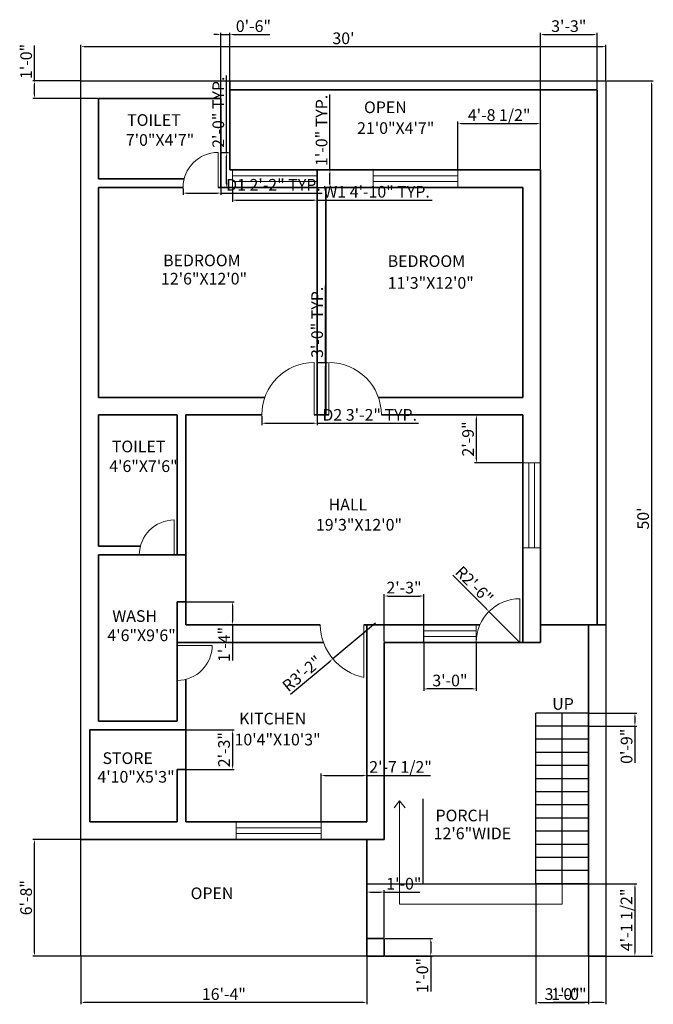
# Model space of a CAD drawing. Units: inches. Extents: x 2514 to 2949, y 1604 to 2279.
import ezdxf

# ---------------------------------------------------------------- set-up
doc = ezdxf.new("R2010")
doc.units = ezdxf.units.IN
for name, color, linetype, lineweight in [('A-ANNO-DIMS', 7, 'Continuous', 18), ('A-ANNO-SYMB', 121, 'Continuous', 18), ('A-ANNO-TEXT', 231, 'Continuous', 18), ('A-AREA-IDEN', 231, 'Continuous', 18), ('A-COLS', 121, 'Continuous', 35), ('A-DOOR', 2, 'Continuous', 18), ('A-FLOR-STRS', 121, 'Continuous', 25), ('A-GLAZ', 40, 'Continuous', 18), ('A-WALL', 121, 'Continuous', 35), ('C-PROP', 121, 'Continuous', 25)]:
    doc.layers.add(name, color=color, linetype=linetype, lineweight=lineweight)
doc.styles.get("Standard").update_dxf_attribs({"font": 'arial.ttf'})
doc.dimstyles.new('ISO-25', dxfattribs={"dimtxt": 8, "dimasz": 2.5, "dimexe": 1.25, "dimexo": 0.625, "dimtad": 1, "dimdec": 0, "dimlunit": 3, "dimtxsty": 'Standard', "dimcen": 2.5, "dimadec": 0, "dimazin": 0, "dimtfac": 1, "dimtdec": 0, "dimtmove": 0, "dimatfit": 3, "dimfxl": 1, "dimarcsym": 0})

# ---------------------------------------------------------------- blocks, each defined once
blk = doc.blocks.new('*D1')
at = {"layer": 'A-ANNO-DIMS', "color": 0, "lineweight": -2, "transparency": 16777216}
for p, q in [((2556.32, 2237.43), (2556.32, 2261.58)), ((2558.82, 2260.33), (2913.82, 2260.33)), ((2916.32, 2237.43), (2916.32, 2261.58))]:
    blk.add_line(p, q, dxfattribs=at)
at = {"layer": 'A-ANNO-DIMS', "color": 0, "transparency": 16777216}
for points in [[(2558.82, 2260.74), (2558.82, 2259.91), (2556.32, 2260.33)], [(2913.82, 2260.74), (2913.82, 2259.91), (2916.32, 2260.33)]]:
    blk.add_solid(points, dxfattribs=at)
at = {"layer": 'Defpoints', "color": 0, "transparency": 16777216}
for p in [(2916.32, 2260.33), (2556.32, 2236.8), (2916.32, 2236.8)]:
    blk.add_point(p, dxfattribs=at)
at = {"layer": 'A-ANNO-DIMS', "color": 0, "transparency": 16777216, "insert": (2736.32, 2265.04), "char_height": 8, "attachment_point": 5}
blk.add_mtext("30'", dxfattribs=at)
blk = doc.blocks.new('*D2')
at = {"layer": 'A-ANNO-DIMS', "color": 0, "lineweight": -2, "transparency": 16777216}
for p, q in [((2916.94, 2236.8), (2948.78, 2236.8)), ((2947.53, 2234.3), (2947.53, 1639.3)), ((2916.94, 1636.8), (2948.78, 1636.8))]:
    blk.add_line(p, q, dxfattribs=at)
at = {"layer": 'A-ANNO-DIMS', "color": 0, "transparency": 16777216}
for points in [[(2947.11, 2234.3), (2947.95, 2234.3), (2947.53, 2236.8)], [(2947.11, 1639.3), (2947.95, 1639.3), (2947.53, 1636.8)]]:
    blk.add_solid(points, dxfattribs=at)
at = {"layer": 'Defpoints', "color": 0, "transparency": 16777216}
for p in [(2916.32, 2236.8), (2916.32, 1636.8), (2947.53, 1636.8)]:
    blk.add_point(p, dxfattribs=at)
at = {"layer": 'A-ANNO-DIMS', "color": 0, "transparency": 16777216, "insert": (2942.82, 1936.8), "char_height": 8, "attachment_point": 5, "rotation": 90}
blk.add_mtext("50'", dxfattribs=at)
blk = doc.blocks.new('DOOR-SWING-24IN')
for p, q in [((0, 0), (0, 24)), ((2, 0), (0, 0))]:
    blk.add_line(p, q)
blk.add_arc((0, 0), 24, 90, 180)
blk = doc.blocks.new('DOOR-SWING-36IN')
for p, q in [((0, 0), (0, 36)), ((2, 0), (0, 0))]:
    blk.add_line(p, q)
blk.add_arc((0, 0), 36, 90, 180)
blk = doc.blocks.new('WIN-WIDE-12IN-WALL')
for p, q in [((0, 12), (0, 0)), ((0, 8), (58.18, 8)), ((58.18, 0), (58.18, 12)), ((0, 4), (58.18, 4))]:
    blk.add_line(p, q)
blk = doc.blocks.new('STAIR-TREAD-36IN')
for p, q in [((18, 0), (0, 0)), ((36, 0), (18, 0))]:
    blk.add_line(p, q)
blk = doc.blocks.new('*D7')
at = {"layer": 'A-ANNO-DIMS', "color": 0, "lineweight": -2, "transparency": 16777216}
for p, q in [((2660.14, 2163.18), (2660.14, 2153.83)), ((2718.32, 2163.18), (2718.32, 2153.83)), ((2662.64, 2155.08), (2715.82, 2155.08)), ((2718.32, 2155.08), (2797.24, 2155.08))]:
    blk.add_line(p, q, dxfattribs=at)
at = {"layer": 'A-ANNO-DIMS', "color": 0, "transparency": 16777216}
for points in [[(2662.64, 2155.49), (2662.64, 2154.66), (2660.14, 2155.08)], [(2715.82, 2155.49), (2715.82, 2154.66), (2718.32, 2155.08)]]:
    blk.add_solid(points, dxfattribs=at)
at = {"layer": 'Defpoints', "color": 0, "transparency": 16777216}
for p in [(2660.14, 2163.8), (2718.32, 2163.8), (2718.32, 2155.08)]:
    blk.add_point(p, dxfattribs=at)
at = {"layer": 'A-ANNO-DIMS', "color": 0, "transparency": 16777216, "insert": (2759.03, 2159.79), "char_height": 8, "attachment_point": 5}
blk.add_mtext('W1 4\'-10" TYP.', dxfattribs=at)
blk = doc.blocks.new('*D8')
at = {"layer": 'A-ANNO-DIMS', "color": 0, "lineweight": -2, "transparency": 16777216}
for p, q in [((2727.04, 2175.8), (2727.04, 2227.56)), ((2718.94, 2175.8), (2728.29, 2175.8)), ((2727.04, 2166.3), (2727.04, 2173.3)), ((2718.94, 2163.8), (2728.29, 2163.8))]:
    blk.add_line(p, q, dxfattribs=at)
at = {"layer": 'A-ANNO-DIMS', "color": 0, "transparency": 16777216}
for points in [[(2726.62, 2173.3), (2727.46, 2173.3), (2727.04, 2175.8)], [(2726.62, 2166.3), (2727.46, 2166.3), (2727.04, 2163.8)]]:
    blk.add_solid(points, dxfattribs=at)
at = {"layer": 'Defpoints', "color": 0, "transparency": 16777216}
for p in [(2718.32, 2175.8), (2727.04, 2175.8), (2718.32, 2163.8)]:
    blk.add_point(p, dxfattribs=at)
at = {"layer": 'A-ANNO-DIMS', "color": 0, "transparency": 16777216, "insert": (2722.33, 2202.93), "char_height": 8, "attachment_point": 5, "rotation": 90}
blk.add_mtext('1\'-0" TYP.', dxfattribs=at)
blk = doc.blocks.new('*D9')
at = {"layer": 'A-ANNO-DIMS', "color": 0, "lineweight": -2, "transparency": 16777216}
for p, q in [((2626.32, 2163.18), (2626.32, 2158.65)), ((2652.32, 2163.18), (2652.32, 2158.65)), ((2628.82, 2159.9), (2649.82, 2159.9)), ((2652.32, 2159.9), (2721.82, 2159.9))]:
    blk.add_line(p, q, dxfattribs=at)
at = {"layer": 'A-ANNO-DIMS', "color": 0, "transparency": 16777216}
for points in [[(2628.82, 2160.32), (2628.82, 2159.49), (2626.32, 2159.9)], [(2649.82, 2160.32), (2649.82, 2159.49), (2652.32, 2159.9)]]:
    blk.add_solid(points, dxfattribs=at)
at = {"layer": 'Defpoints', "color": 0, "transparency": 16777216}
for p in [(2626.32, 2163.8), (2652.32, 2163.8), (2652.32, 2159.9)]:
    blk.add_point(p, dxfattribs=at)
at = {"layer": 'A-ANNO-DIMS', "color": 0, "transparency": 16777216, "insert": (2688.32, 2164.55), "char_height": 8, "attachment_point": 5}
blk.add_mtext('D1 2\'-2" TYP.', dxfattribs=at)
blk = doc.blocks.new('*D10')
at = {"layer": 'A-ANNO-DIMS', "color": 0, "lineweight": -2, "transparency": 16777216}
for p, q in [((2656.22, 2187.8), (2656.22, 2240.45)), ((2652.94, 2187.8), (2657.47, 2187.8)), ((2656.22, 2166.3), (2656.22, 2185.3)), ((2652.94, 2163.8), (2657.47, 2163.8))]:
    blk.add_line(p, q, dxfattribs=at)
at = {"layer": 'A-ANNO-DIMS', "color": 0, "transparency": 16777216}
for points in [[(2655.8, 2185.3), (2656.63, 2185.3), (2656.22, 2187.8)], [(2655.8, 2166.3), (2656.63, 2166.3), (2656.22, 2163.8)]]:
    blk.add_solid(points, dxfattribs=at)
at = {"layer": 'Defpoints', "color": 0, "transparency": 16777216}
for p in [(2652.32, 2187.8), (2656.22, 2187.8), (2652.32, 2163.8)]:
    blk.add_point(p, dxfattribs=at)
at = {"layer": 'A-ANNO-DIMS', "color": 0, "transparency": 16777216, "insert": (2651.51, 2215.38), "char_height": 8, "attachment_point": 5, "rotation": 90}
blk.add_mtext('2\'-0" TYP.', dxfattribs=at)
blk = doc.blocks.new('*D11')
at = {"layer": 'A-ANNO-DIMS', "color": 0, "lineweight": -2, "transparency": 16777216}
for p, q in [((2680.32, 2007.18), (2680.32, 2000.85)), ((2718.32, 2007.18), (2718.32, 2000.85)), ((2682.82, 2002.1), (2715.82, 2002.1)), ((2718.32, 2002.1), (2787.82, 2002.1))]:
    blk.add_line(p, q, dxfattribs=at)
at = {"layer": 'A-ANNO-DIMS', "color": 0, "transparency": 16777216}
for points in [[(2682.82, 2002.52), (2682.82, 2001.69), (2680.32, 2002.1)], [(2715.82, 2002.52), (2715.82, 2001.69), (2718.32, 2002.1)]]:
    blk.add_solid(points, dxfattribs=at)
at = {"layer": 'Defpoints', "color": 0, "transparency": 16777216}
for p in [(2680.32, 2007.8), (2718.32, 2007.8), (2718.32, 2002.1)]:
    blk.add_point(p, dxfattribs=at)
at = {"layer": 'A-ANNO-DIMS', "color": 0, "transparency": 16777216, "insert": (2754.32, 2006.82), "char_height": 8, "attachment_point": 5}
blk.add_mtext('D2 3\'-2" TYP.', dxfattribs=at)
blk = doc.blocks.new('*D12')
at = {"layer": 'A-ANNO-DIMS', "color": 0, "lineweight": -2, "transparency": 16777216}
for p, q in [((2724.02, 2043.8), (2724.02, 2096.31)), ((2718.94, 2043.8), (2725.27, 2043.8)), ((2724.02, 2010.3), (2724.02, 2041.3)), ((2718.94, 2007.8), (2725.27, 2007.8))]:
    blk.add_line(p, q, dxfattribs=at)
at = {"layer": 'A-ANNO-DIMS', "color": 0, "transparency": 16777216}
for points in [[(2723.6, 2041.3), (2724.43, 2041.3), (2724.02, 2043.8)], [(2723.6, 2010.3), (2724.43, 2010.3), (2724.02, 2007.8)]]:
    blk.add_solid(points, dxfattribs=at)
at = {"layer": 'Defpoints', "color": 0, "transparency": 16777216}
for p in [(2718.32, 2043.8), (2724.02, 2043.8), (2718.32, 2007.8)]:
    blk.add_point(p, dxfattribs=at)
at = {"layer": 'A-ANNO-DIMS', "color": 0, "transparency": 16777216, "insert": (2719.3, 2071.31), "char_height": 8, "attachment_point": 5, "rotation": 90}
blk.add_mtext('3\'-0" TYP.', dxfattribs=at)
blk = doc.blocks.new('*D13')
at = {"layer": 'A-ANNO-DIMS', "color": 0, "lineweight": -2, "transparency": 16777216}
for p, q in [((2524.47, 2236.8), (2524.47, 2261.07)), ((2555.69, 2236.8), (2523.22, 2236.8)), ((2524.47, 2227.3), (2524.47, 2234.3)), ((2567.69, 2224.8), (2523.22, 2224.8))]:
    blk.add_line(p, q, dxfattribs=at)
at = {"layer": 'A-ANNO-DIMS', "color": 0, "transparency": 16777216}
for points in [[(2524.05, 2234.3), (2524.88, 2234.3), (2524.47, 2236.8)], [(2524.05, 2227.3), (2524.88, 2227.3), (2524.47, 2224.8)]]:
    blk.add_solid(points, dxfattribs=at)
at = {"layer": 'Defpoints', "color": 0, "transparency": 16777216}
for p in [(2524.47, 2236.8), (2556.32, 2236.8), (2568.32, 2224.8)]:
    blk.add_point(p, dxfattribs=at)
at = {"layer": 'A-ANNO-DIMS', "color": 0, "transparency": 16777216, "insert": (2519.76, 2250.18), "char_height": 8, "attachment_point": 5, "rotation": 90}
blk.add_mtext('1\'-0"', dxfattribs=at)
blk = doc.blocks.new('*D14')
at = {"layer": 'A-ANNO-DIMS', "color": 0, "lineweight": -2, "transparency": 16777216}
for p, q in [((2555.69, 1716.8), (2523.22, 1716.8)), ((2524.47, 1639.3), (2524.47, 1714.3)), ((2555.69, 1636.8), (2523.22, 1636.8))]:
    blk.add_line(p, q, dxfattribs=at)
at = {"layer": 'A-ANNO-DIMS', "color": 0, "transparency": 16777216}
for points in [[(2524.05, 1714.3), (2524.88, 1714.3), (2524.47, 1716.8)], [(2524.05, 1639.3), (2524.88, 1639.3), (2524.47, 1636.8)]]:
    blk.add_solid(points, dxfattribs=at)
at = {"layer": 'Defpoints', "color": 0, "transparency": 16777216}
for p in [(2524.47, 1716.8), (2556.32, 1716.8), (2556.32, 1636.8)]:
    blk.add_point(p, dxfattribs=at)
at = {"layer": 'A-ANNO-DIMS', "color": 0, "transparency": 16777216, "insert": (2519.76, 1676.8), "char_height": 8, "attachment_point": 5, "rotation": 90}
blk.add_mtext('6\'-8"', dxfattribs=at)
blk = doc.blocks.new('*D15')
at = {"layer": 'A-ANNO-DIMS', "color": 0, "lineweight": -2, "transparency": 16777216}
for p, q in [((2904.94, 1686.39), (2937.42, 1686.39)), ((2936.17, 1683.89), (2936.17, 1639.3)), ((2904.94, 1636.8), (2937.42, 1636.8))]:
    blk.add_line(p, q, dxfattribs=at)
at = {"layer": 'A-ANNO-DIMS', "color": 0, "transparency": 16777216}
for points in [[(2935.75, 1683.89), (2936.58, 1683.89), (2936.17, 1686.39)], [(2935.75, 1639.3), (2936.58, 1639.3), (2936.17, 1636.8)]]:
    blk.add_solid(points, dxfattribs=at)
at = {"layer": 'Defpoints', "color": 0, "transparency": 16777216}
for p in [(2904.32, 1686.39), (2904.32, 1636.8), (2936.17, 1636.8)]:
    blk.add_point(p, dxfattribs=at)
at = {"layer": 'A-ANNO-DIMS', "color": 0, "transparency": 16777216, "insert": (2931.4, 1661.6), "char_height": 8, "attachment_point": 5, "rotation": 90}
blk.add_mtext('4\'-1 1/2"', dxfattribs=at)
blk = doc.blocks.new('*D16')
at = {"layer": 'A-ANNO-DIMS', "color": 0, "lineweight": -2, "transparency": 16777216}
for p, q in [((2904.94, 1803.39), (2937.42, 1803.39)), ((2936.17, 1800.89), (2936.17, 1796.89)), ((2904.94, 1794.39), (2937.42, 1794.39)), ((2936.17, 1794.39), (2936.17, 1769.38))]:
    blk.add_line(p, q, dxfattribs=at)
at = {"layer": 'A-ANNO-DIMS', "color": 0, "transparency": 16777216}
for points in [[(2935.75, 1800.89), (2936.58, 1800.89), (2936.17, 1803.39)], [(2935.75, 1796.89), (2936.58, 1796.89), (2936.17, 1794.39)]]:
    blk.add_solid(points, dxfattribs=at)
at = {"layer": 'Defpoints', "color": 0, "transparency": 16777216}
for p in [(2904.32, 1803.39), (2904.32, 1794.39), (2936.17, 1794.39)]:
    blk.add_point(p, dxfattribs=at)
at = {"layer": 'A-ANNO-DIMS', "color": 0, "transparency": 16777216, "insert": (2931.46, 1780.63), "char_height": 8, "attachment_point": 5, "rotation": 90}
blk.add_mtext('0\'-9"', dxfattribs=at)
blk = doc.blocks.new('*D17')
at = {"layer": 'A-ANNO-DIMS', "color": 0, "lineweight": -2, "transparency": 16777216}
for p, q in [((2868.32, 1685.77), (2868.32, 1603.7)), ((2904.32, 1685.77), (2904.32, 1603.7)), ((2870.82, 1604.95), (2901.82, 1604.95))]:
    blk.add_line(p, q, dxfattribs=at)
at = {"layer": 'A-ANNO-DIMS', "color": 0, "transparency": 16777216}
for points in [[(2870.82, 1605.37), (2870.82, 1604.54), (2868.32, 1604.95)], [(2901.82, 1605.37), (2901.82, 1604.54), (2904.32, 1604.95)]]:
    blk.add_solid(points, dxfattribs=at)
at = {"layer": 'Defpoints', "color": 0, "transparency": 16777216}
for p in [(2868.32, 1686.39), (2904.32, 1686.39), (2904.32, 1604.95)]:
    blk.add_point(p, dxfattribs=at)
at = {"layer": 'A-ANNO-DIMS', "color": 0, "transparency": 16777216, "insert": (2886.32, 1609.67), "char_height": 8, "attachment_point": 5}
blk.add_mtext('3\'-0"', dxfattribs=at)
blk = doc.blocks.new('*D18')
at = {"layer": 'A-ANNO-DIMS', "color": 0, "lineweight": -2, "transparency": 16777216}
for p, q in [((2904.32, 1636.18), (2904.32, 1603.7)), ((2916.32, 1636.18), (2916.32, 1603.7)), ((2904.32, 1604.95), (2880.05, 1604.95)), ((2913.82, 1604.95), (2906.82, 1604.95))]:
    blk.add_line(p, q, dxfattribs=at)
at = {"layer": 'A-ANNO-DIMS', "color": 0, "transparency": 16777216}
for points in [[(2906.82, 1605.37), (2906.82, 1604.54), (2904.32, 1604.95)], [(2913.82, 1605.37), (2913.82, 1604.54), (2916.32, 1604.95)]]:
    blk.add_solid(points, dxfattribs=at)
at = {"layer": 'Defpoints', "color": 0, "transparency": 16777216}
for p in [(2904.32, 1636.8), (2916.32, 1636.8), (2904.32, 1604.95)]:
    blk.add_point(p, dxfattribs=at)
at = {"layer": 'A-ANNO-DIMS', "color": 0, "transparency": 16777216, "insert": (2890.93, 1609.66), "char_height": 8, "attachment_point": 5}
blk.add_mtext('1\'-0"', dxfattribs=at)
blk = doc.blocks.new('*D19')
at = {"layer": 'A-ANNO-DIMS', "color": 0, "lineweight": -2, "transparency": 16777216}
for p, q in [((2556.32, 1636.18), (2556.32, 1603.7)), ((2752.32, 1636.18), (2752.32, 1603.7)), ((2749.82, 1604.95), (2558.82, 1604.95))]:
    blk.add_line(p, q, dxfattribs=at)
at = {"layer": 'A-ANNO-DIMS', "color": 0, "transparency": 16777216}
for points in [[(2558.82, 1605.37), (2558.82, 1604.54), (2556.32, 1604.95)], [(2749.82, 1605.37), (2749.82, 1604.54), (2752.32, 1604.95)]]:
    blk.add_solid(points, dxfattribs=at)
at = {"layer": 'Defpoints', "color": 0, "transparency": 16777216}
for p in [(2556.32, 1636.8), (2752.32, 1636.8), (2556.32, 1604.95)]:
    blk.add_point(p, dxfattribs=at)
at = {"layer": 'A-ANNO-DIMS', "color": 0, "transparency": 16777216, "insert": (2654.32, 1609.66), "char_height": 8, "attachment_point": 5}
blk.add_mtext('16\'-4"', dxfattribs=at)
blk = doc.blocks.new('*D20')
at = {"layer": 'A-ANNO-DIMS', "color": 0, "lineweight": -2, "transparency": 16777216}
for p, q in [((2871.32, 2176.43), (2871.32, 2269.9)), ((2873.82, 2268.65), (2907.82, 2268.65)), ((2910.32, 2231.43), (2910.32, 2269.9))]:
    blk.add_line(p, q, dxfattribs=at)
at = {"layer": 'A-ANNO-DIMS', "color": 0, "transparency": 16777216}
for points in [[(2873.82, 2269.07), (2873.82, 2268.24), (2871.32, 2268.65)], [(2907.82, 2269.07), (2907.82, 2268.24), (2910.32, 2268.65)]]:
    blk.add_solid(points, dxfattribs=at)
at = {"layer": 'Defpoints', "color": 0, "transparency": 16777216}
for p in [(2910.32, 2268.65), (2910.32, 2230.8), (2871.32, 2175.8)]:
    blk.add_point(p, dxfattribs=at)
at = {"layer": 'A-ANNO-DIMS', "color": 0, "transparency": 16777216, "insert": (2890.82, 2273.37), "char_height": 8, "attachment_point": 5}
blk.add_mtext('3\'-3"', dxfattribs=at)
blk = doc.blocks.new('*D21')
at = {"layer": 'A-ANNO-DIMS', "color": 0, "lineweight": -2, "transparency": 16777216}
for p, q in [((2721.03, 1729.43), (2721.03, 1761.9)), ((2723.53, 1760.65), (2749.82, 1760.65)), ((2752.32, 1729.43), (2752.32, 1761.9)), ((2752.32, 1760.65), (2796.11, 1760.65))]:
    blk.add_line(p, q, dxfattribs=at)
at = {"layer": 'A-ANNO-DIMS', "color": 0, "transparency": 16777216}
for points in [[(2723.53, 1761.07), (2723.53, 1760.24), (2721.03, 1760.65)], [(2749.82, 1761.07), (2749.82, 1760.24), (2752.32, 1760.65)]]:
    blk.add_solid(points, dxfattribs=at)
at = {"layer": 'Defpoints', "color": 0, "transparency": 16777216}
for p in [(2752.32, 1760.65), (2721.03, 1728.8), (2752.32, 1728.8)]:
    blk.add_point(p, dxfattribs=at)
at = {"layer": 'A-ANNO-DIMS', "color": 0, "transparency": 16777216, "insert": (2775.46, 1765.41), "char_height": 8, "attachment_point": 5}
blk.add_mtext('2\'-7 1/2"', dxfattribs=at)
blk = doc.blocks.new('*D22')
at = {"layer": 'A-ANNO-DIMS', "color": 0, "lineweight": -2, "transparency": 16777216}
for p, q in [((2858.69, 2007.8), (2826.22, 2007.8)), ((2827.47, 1977.38), (2827.47, 2005.3)), ((2858.69, 1974.88), (2826.22, 1974.88))]:
    blk.add_line(p, q, dxfattribs=at)
at = {"layer": 'A-ANNO-DIMS', "color": 0, "transparency": 16777216}
for points in [[(2827.05, 2005.3), (2827.88, 2005.3), (2827.47, 2007.8)], [(2827.05, 1977.38), (2827.88, 1977.38), (2827.47, 1974.88)]]:
    blk.add_solid(points, dxfattribs=at)
at = {"layer": 'Defpoints', "color": 0, "transparency": 16777216}
for p in [(2827.47, 2007.8), (2859.32, 2007.8), (2859.32, 1974.88)]:
    blk.add_point(p, dxfattribs=at)
at = {"layer": 'A-ANNO-DIMS', "color": 0, "transparency": 16777216, "insert": (2822.76, 1991.34), "char_height": 8, "attachment_point": 5, "rotation": 90}
blk.add_mtext('2\'-9"', dxfattribs=at)
blk = doc.blocks.new('*D23')
at = {"layer": 'A-ANNO-DIMS', "color": 0, "lineweight": -2, "transparency": 16777216}
for p, q in [((2814.84, 2176.43), (2814.84, 2208.9)), ((2817.34, 2207.65), (2868.82, 2207.65)), ((2871.32, 2176.43), (2871.32, 2208.9))]:
    blk.add_line(p, q, dxfattribs=at)
at = {"layer": 'A-ANNO-DIMS', "color": 0, "transparency": 16777216}
for points in [[(2817.34, 2208.07), (2817.34, 2207.24), (2814.84, 2207.65)], [(2868.82, 2208.07), (2868.82, 2207.24), (2871.32, 2207.65)]]:
    blk.add_solid(points, dxfattribs=at)
at = {"layer": 'Defpoints', "color": 0, "transparency": 16777216}
for p in [(2871.32, 2207.65), (2814.84, 2175.8), (2871.32, 2175.8)]:
    blk.add_point(p, dxfattribs=at)
at = {"layer": 'A-ANNO-DIMS', "color": 0, "transparency": 16777216, "insert": (2843.08, 2212.41), "char_height": 8, "attachment_point": 5}
blk.add_mtext('4\'-8 1/2"', dxfattribs=at)
blk = doc.blocks.new('*D24')
at = {"layer": 'A-ANNO-DIMS', "color": 0, "lineweight": -2, "transparency": 16777216}
for p, q in [((2649.82, 2268.65), (2647.32, 2268.65)), ((2652.32, 2225.43), (2652.32, 2269.9)), ((2652.32, 2268.65), (2658.32, 2268.65)), ((2658.32, 2237.43), (2658.32, 2269.9)), ((2660.82, 2268.65), (2685.83, 2268.65))]:
    blk.add_line(p, q, dxfattribs=at)
at = {"layer": 'A-ANNO-DIMS', "color": 0, "transparency": 16777216}
for points in [[(2649.82, 2269.07), (2649.82, 2268.24), (2652.32, 2268.65)], [(2660.82, 2269.07), (2660.82, 2268.24), (2658.32, 2268.65)]]:
    blk.add_solid(points, dxfattribs=at)
at = {"layer": 'Defpoints', "color": 0, "transparency": 16777216}
for p in [(2658.32, 2268.65), (2658.32, 2236.8), (2652.32, 2224.8)]:
    blk.add_point(p, dxfattribs=at)
at = {"layer": 'A-ANNO-DIMS', "color": 0, "transparency": 16777216, "insert": (2674.57, 2273.36), "char_height": 8, "attachment_point": 5}
blk.add_mtext('0\'-6"', dxfattribs=at)
blk = doc.blocks.new('*D25')
at = {"layer": 'A-ANNO-DIMS', "color": 0, "lineweight": -2, "transparency": 16777216}
for p, q in [((2791.32, 1851.18), (2791.32, 1818.7)), ((2827.32, 1851.18), (2827.32, 1818.7)), ((2824.82, 1819.95), (2793.82, 1819.95))]:
    blk.add_line(p, q, dxfattribs=at)
at = {"layer": 'A-ANNO-DIMS', "color": 0, "transparency": 16777216}
for points in [[(2793.82, 1820.37), (2793.82, 1819.54), (2791.32, 1819.95)], [(2824.82, 1820.37), (2824.82, 1819.54), (2827.32, 1819.95)]]:
    blk.add_solid(points, dxfattribs=at)
at = {"layer": 'Defpoints', "color": 0, "transparency": 16777216}
for p in [(2791.32, 1851.8), (2827.32, 1851.8), (2791.32, 1819.95)]:
    blk.add_point(p, dxfattribs=at)
at = {"layer": 'A-ANNO-DIMS', "color": 0, "transparency": 16777216, "insert": (2809.32, 1824.67), "char_height": 8, "attachment_point": 5}
blk.add_mtext('3\'-0"', dxfattribs=at)
blk = doc.blocks.new('*D26')
at = {"layer": 'A-ANNO-DIMS', "color": 0, "lineweight": -2, "transparency": 16777216}
for p, q in [((2764.32, 1852.43), (2764.32, 1884.9)), ((2766.82, 1883.65), (2788.82, 1883.65)), ((2791.32, 1852.43), (2791.32, 1884.9))]:
    blk.add_line(p, q, dxfattribs=at)
at = {"layer": 'A-ANNO-DIMS', "color": 0, "transparency": 16777216}
for points in [[(2766.82, 1884.07), (2766.82, 1883.24), (2764.32, 1883.65)], [(2788.82, 1884.07), (2788.82, 1883.24), (2791.32, 1883.65)]]:
    blk.add_solid(points, dxfattribs=at)
at = {"layer": 'Defpoints', "color": 0, "transparency": 16777216}
for p in [(2791.32, 1883.65), (2764.32, 1851.8), (2791.32, 1851.8)]:
    blk.add_point(p, dxfattribs=at)
at = {"layer": 'A-ANNO-DIMS', "color": 0, "transparency": 16777216, "insert": (2777.82, 1888.37), "char_height": 8, "attachment_point": 5}
blk.add_mtext('2\'-3"', dxfattribs=at)
blk = doc.blocks.new('*D27')
at = {"layer": 'A-ANNO-DIMS', "color": 0, "lineweight": -2, "transparency": 16777216}
for p, q in [((2628.94, 1879.73), (2661.42, 1879.73)), ((2660.17, 1877.23), (2660.17, 1866.3)), ((2628.94, 1863.8), (2661.42, 1863.8)), ((2660.17, 1863.8), (2660.17, 1839.54))]:
    blk.add_line(p, q, dxfattribs=at)
at = {"layer": 'A-ANNO-DIMS', "color": 0, "transparency": 16777216}
for points in [[(2659.75, 1877.23), (2660.58, 1877.23), (2660.17, 1879.73)], [(2659.75, 1866.3), (2660.58, 1866.3), (2660.17, 1863.8)]]:
    blk.add_solid(points, dxfattribs=at)
at = {"layer": 'Defpoints', "color": 0, "transparency": 16777216}
for p in [(2628.32, 1879.73), (2628.32, 1863.8), (2660.17, 1863.8)]:
    blk.add_point(p, dxfattribs=at)
at = {"layer": 'A-ANNO-DIMS', "color": 0, "transparency": 16777216, "insert": (2655.52, 1850.42), "char_height": 8, "attachment_point": 5, "rotation": 90}
blk.add_mtext('1\'-4"', dxfattribs=at)
blk = doc.blocks.new('*D28')
at = {"layer": 'A-ANNO-DIMS', "color": 0, "lineweight": -2, "transparency": 16777216}
for p, q in [((2628.94, 1791.8), (2661.42, 1791.8)), ((2660.17, 1789.3), (2660.17, 1767.3)), ((2628.94, 1764.8), (2661.42, 1764.8))]:
    blk.add_line(p, q, dxfattribs=at)
at = {"layer": 'A-ANNO-DIMS', "color": 0, "transparency": 16777216}
for points in [[(2659.75, 1789.3), (2660.58, 1789.3), (2660.17, 1791.8)], [(2659.75, 1767.3), (2660.58, 1767.3), (2660.17, 1764.8)]]:
    blk.add_solid(points, dxfattribs=at)
at = {"layer": 'Defpoints', "color": 0, "transparency": 16777216}
for p in [(2628.32, 1791.8), (2628.32, 1764.8), (2660.17, 1764.8)]:
    blk.add_point(p, dxfattribs=at)
at = {"layer": 'A-ANNO-DIMS', "color": 0, "transparency": 16777216, "insert": (2655.45, 1778.3), "char_height": 8, "attachment_point": 5, "rotation": 90}
blk.add_mtext('2\'-3"', dxfattribs=at)
blk = doc.blocks.new('*D29')
at = {"layer": 'A-ANNO-DIMS', "color": 0, "lineweight": -2, "transparency": 16777216}
for p, q in [((2752.32, 1649.43), (2752.32, 1681.9)), ((2764.32, 1649.43), (2764.32, 1681.9)), ((2754.82, 1680.65), (2761.82, 1680.65)), ((2764.32, 1680.65), (2788.58, 1680.65))]:
    blk.add_line(p, q, dxfattribs=at)
at = {"layer": 'A-ANNO-DIMS', "color": 0, "transparency": 16777216}
for points in [[(2754.82, 1681.07), (2754.82, 1680.24), (2752.32, 1680.65)], [(2761.82, 1681.07), (2761.82, 1680.24), (2764.32, 1680.65)]]:
    blk.add_solid(points, dxfattribs=at)
at = {"layer": 'Defpoints', "color": 0, "transparency": 16777216}
for p in [(2764.32, 1680.65), (2752.32, 1648.8), (2764.32, 1648.8)]:
    blk.add_point(p, dxfattribs=at)
at = {"layer": 'A-ANNO-DIMS', "color": 0, "transparency": 16777216, "insert": (2777.7, 1685.36), "char_height": 8, "attachment_point": 5}
blk.add_mtext('1\'-0"', dxfattribs=at)
blk = doc.blocks.new('*D30')
at = {"layer": 'A-ANNO-DIMS', "color": 0, "lineweight": -2, "transparency": 16777216}
for p, q in [((2764.94, 1648.8), (2797.42, 1648.8)), ((2796.17, 1646.3), (2796.17, 1639.3)), ((2764.94, 1636.8), (2797.42, 1636.8)), ((2796.17, 1636.8), (2796.17, 1612.54))]:
    blk.add_line(p, q, dxfattribs=at)
at = {"layer": 'A-ANNO-DIMS', "color": 0, "transparency": 16777216}
for points in [[(2795.75, 1646.3), (2796.58, 1646.3), (2796.17, 1648.8)], [(2795.75, 1639.3), (2796.58, 1639.3), (2796.17, 1636.8)]]:
    blk.add_solid(points, dxfattribs=at)
at = {"layer": 'Defpoints', "color": 0, "transparency": 16777216}
for p in [(2764.32, 1648.8), (2764.32, 1636.8), (2796.17, 1636.8)]:
    blk.add_point(p, dxfattribs=at)
at = {"layer": 'A-ANNO-DIMS', "color": 0, "transparency": 16777216, "insert": (2791.46, 1623.42), "char_height": 8, "attachment_point": 5, "rotation": 90}
blk.add_mtext('1\'-0"', dxfattribs=at)
blk = doc.blocks.new('*D31')
at = {"layer": 'A-ANNO-DIMS', "color": 0, "lineweight": -2, "transparency": 16777216}
for p, q in [((2758.3, 1864.96), (2729.11, 1840.63)), ((2700, 1816.37), (2727.18, 1839.03))]:
    blk.add_line(p, q, dxfattribs=at)
at = {"layer": 'A-ANNO-DIMS', "color": 0, "transparency": 16777216}
blk.add_solid([(2726.92, 1839.35), (2727.45, 1838.71), (2729.11, 1840.63)], dxfattribs=at)
at = {"layer": 'Defpoints', "color": 0, "transparency": 16777216}
for p in [(2758.3, 1864.96), (2729.11, 1840.63)]:
    blk.add_point(p, dxfattribs=at)
at = {"layer": 'A-ANNO-DIMS', "color": 0, "transparency": 16777216, "insert": (2708.57, 1829.65), "char_height": 8, "attachment_point": 5, "rotation": 39.80561}
blk.add_mtext('R3\'-2"', dxfattribs=at)
blk = doc.blocks.new('*D32')
at = {"layer": 'A-ANNO-DIMS', "color": 0, "lineweight": -2, "transparency": 16777216}
for p, q in [((2811.23, 1897.89), (2834.33, 1874.78)), ((2857.32, 1851.8), (2836.1, 1873.02))]:
    blk.add_line(p, q, dxfattribs=at)
at = {"layer": 'A-ANNO-DIMS', "color": 0, "transparency": 16777216}
blk.add_solid([(2834.63, 1875.08), (2834.04, 1874.49), (2836.1, 1873.02)], dxfattribs=at)
at = {"layer": 'Defpoints', "color": 0, "transparency": 16777216}
for p in [(2836.1, 1873.02), (2857.32, 1851.8)]:
    blk.add_point(p, dxfattribs=at)
at = {"layer": 'A-ANNO-DIMS', "color": 0, "transparency": 16777216, "insert": (2825.23, 1890.55), "char_height": 8, "attachment_point": 5, "rotation": 315.00022}
blk.add_mtext('R2\'-6"', dxfattribs=at)

msp = doc.modelspace()

# ---------------------------------------------------------------- linework, layer by layer
at = {"layer": 'A-ANNO-SYMB'}
for p, q in [((2774.84, 1743.11), (2770.99, 1738.52)), ((2774.84, 1672.39), (2774.84, 1743.11)), ((2774.84, 1743.11), (2778.7, 1738.52)), ((2886.32, 1686.39), (2886.32, 1672.39)), ((2886.32, 1672.39), (2774.84, 1672.39))]:
    msp.add_line(p, q, dxfattribs=at)
at = {"layer": 'A-COLS'}
for p, q in [((2764.32, 1648.8), (2752.32, 1648.8)), ((2764.32, 1636.8), (2764.32, 1648.8)), ((2752.32, 1636.8), (2764.32, 1636.8))]:
    msp.add_line(p, q, dxfattribs=at)
at = {"layer": 'A-DOOR'}
for p, q in [((2857.32, 1851.8), (2857.32, 1881.8)), ((2752.32, 1863.8), (2750.32, 1863.8)), ((2750.32, 1863.8), (2750.32, 1827.8)), ((2859.32, 1851.8), (2857.32, 1851.8))]:
    msp.add_line(p, q, dxfattribs=at)
for centre, radius, start, end in [((2857.32, 1851.8), 30, 90, 180), ((2758.3, 1864.96), 38, 181.7374, 257.87374)]:
    msp.add_arc(centre, radius, start, end, dxfattribs=at)
at = {"layer": 'A-FLOR-STRS'}
for p, q in [((2868.32, 1686.39), (2868.32, 1803.39)), ((2886.32, 1686.39), (2886.32, 1803.39)), ((2790.95, 1686.39), (2790.95, 1744.49)), ((2752.32, 1686.39), (2904.32, 1686.39))]:
    msp.add_line(p, q, dxfattribs=at)
at = {"layer": 'A-GLAZ'}
for p, q in [((2791.32, 1851.8), (2791.32, 1863.8)), ((2827.32, 1851.8), (2827.32, 1863.8)), ((2791.32, 1859.8), (2827.32, 1859.8)), ((2791.32, 1855.8), (2827.32, 1855.8))]:
    msp.add_line(p, q, dxfattribs=at)
at = {"layer": 'A-WALL'}
for p, q in [((2658.32, 2175.8), (2658.32, 2236.8)), ((2658.32, 2230.8), (2910.32, 2230.8)), ((2910.32, 2230.8), (2910.32, 1863.8)), ((2568.32, 2224.8), (2652.32, 2224.8)), ((2568.32, 2169.8), (2568.32, 2224.8)), ((2652.32, 2163.8), (2652.32, 2224.8)), ((2658.32, 2175.8), (2871.32, 2175.8)), ((2718.32, 2007.8), (2718.32, 2175.8)), ((2871.32, 1851.8), (2871.32, 2175.8)), ((2568.32, 2169.8), (2627.08, 2169.8)), ((2568.32, 2163.8), (2626.32, 2163.8)), ((2568.32, 2019.8), (2568.32, 2163.8)), ((2650.32, 2163.8), (2718.32, 2163.8)), ((2724.32, 2007.8), (2724.32, 2163.8)), ((2724.32, 2163.8), (2859.32, 2163.8)), ((2859.32, 2019.8), (2859.32, 2163.8)), ((2568.32, 2019.8), (2682.37, 2019.8)), ((2760.26, 2019.8), (2859.32, 2019.8)), ((2568.32, 2007.8), (2622.32, 2007.8)), ((2568.32, 1917.8), (2568.32, 2007.8)), ((2622.32, 1911.8), (2622.32, 2007.8)), ((2628.32, 1863.8), (2628.32, 2007.8)), ((2628.32, 2007.8), (2680.32, 2007.8)), ((2716.32, 2007.8), (2724.32, 2007.8)), ((2724.32, 2007.8), (2726.32, 2007.8)), ((2762.32, 2007.8), (2859.32, 2007.8)), ((2859.32, 1851.8), (2859.32, 2007.8)), ((2568.32, 1917.8), (2597.08, 1917.8)), ((2568.32, 1797.8), (2568.32, 1911.8)), ((2568.32, 1911.8), (2628.32, 1911.8)), ((2622.32, 1797.8), (2622.32, 1879.73)), ((2628.32, 1879.73), (2622.32, 1879.73)), ((2628.32, 1863.8), (2720.32, 1863.8)), ((2750.32, 1863.8), (2829.82, 1863.8)), ((2752.32, 1728.8), (2752.32, 1863.8)), ((2871.32, 1863.8), (2916.32, 1863.8)), ((2904.32, 1863.8), (2904.32, 1636.8)), ((2622.32, 1851.8), (2722.65, 1851.8)), ((2764.32, 1716.8), (2764.32, 1851.8)), ((2764.32, 1851.8), (2871.32, 1851.8)), ((2628.32, 1728.8), (2628.32, 1826.57)), ((2568.32, 1797.8), (2622.32, 1797.8)), ((2562.32, 1791.8), (2628.32, 1791.8)), ((2562.32, 1728.8), (2562.32, 1791.8)), ((2622.32, 1728.8), (2622.32, 1764.8)), ((2622.32, 1728.8), (2622.32, 1764.8)), ((2622.32, 1764.8), (2628.32, 1764.8)), ((2562.32, 1728.8), (2622.32, 1728.8)), ((2628.32, 1728.8), (2752.32, 1728.8)), ((2556.32, 1716.8), (2764.32, 1716.8)), ((2752.32, 1636.8), (2752.32, 1716.8))]:
    msp.add_line(p, q, dxfattribs=at)
at = {"layer": 'C-PROP'}
msp.add_lwpolyline([(2556.32, 2236.8), (2916.32, 2236.8), (2916.32, 1636.8), (2556.32, 1636.8)], close=True, dxfattribs=at)

# ---------------------------------------------------------------- block references
at = {"layer": 'A-DOOR'}
for name, p in [('DOOR-SWING-24IN', (2650.32, 2163.8)), ('DOOR-SWING-36IN', (2716.32, 2007.8)), ('DOOR-SWING-24IN', (2620.32, 1911.8))]:
    msp.add_blockref(name, p, dxfattribs=at)
at = {"layer": 'A-DOOR', "extrusion": (0, 0, -1), "zscale": -1}
msp.add_blockref('DOOR-SWING-36IN', (-2726.32, 2007.8), dxfattribs=at)
at = {"layer": 'A-DOOR', "extrusion": (0, 0, -1), "zscale": -1, "rotation": 90.00000000000075}
msp.add_blockref('DOOR-SWING-24IN', (-2622.32, 1849.8), dxfattribs=at)
at = {"layer": 'A-FLOR-STRS'}
for p in [(2868.32, 1803.39), (2868.32, 1794.39), (2868.32, 1785.39), (2868.32, 1776.39), (2868.32, 1767.39), (2868.32, 1758.39), (2868.32, 1749.39), (2868.32, 1740.39), (2868.32, 1731.39), (2868.32, 1722.39), (2868.32, 1713.39), (2868.32, 1704.39), (2868.32, 1695.39), (2868.32, 1686.39)]:
    msp.add_blockref('STAIR-TREAD-36IN', p, dxfattribs=at)
at = {"layer": 'A-GLAZ'}
msp.add_blockref('WIN-WIDE-12IN-WALL', (2660.14, 2163.8), dxfattribs=at)
for p, rotation in [((2814.84, 2175.8), 180), ((2859.32, 1974.88), 270.0000000000007), ((2721.03, 1728.8), 180)]:
    msp.add_blockref('WIN-WIDE-12IN-WALL', p, dxfattribs=dict(at, rotation=rotation))

# ---------------------------------------------------------------- texts
at = {"layer": 'A-ANNO-TEXT'}
msp.add_attdef('UP', (2879.49, 1805.68), '', height=8, dxfattribs=at)
at = {"layer": 'A-AREA-IDEN'}
for tag, p in [('OPEN', (2750.39, 2214.75)), ('TOILET', (2587.98, 2206.01)), ('21\'0"X4\'7"', (2745.68, 2200.49)), ('7\'0"X4\'7"', (2587.07, 2192.35)), ('BEDROOM', (2612.65, 2109.77)), ('BEDROOM', (2766.66, 2109.28)), ('12\'6"X12\'0"', (2611.21, 2097.23)), ('11\'3"X12\'0"', (2766.66, 2094.33)), ('TOILET', (2577.5, 1982.19)), ('4\'6"X7\'6"', (2575.7, 1968.69)), ('HALL', (2726.15, 1942.32)), ('19\'3"X12\'0"', (2717.45, 1928.5)), ('WASH', (2577.81, 1865.91)), ('4\'6"X9\'6"', (2574.43, 1852.7)), ('KITCHEN', (2664.76, 1795.57)), ('10\'4"X10\'3"', (2661.64, 1781.22)), ('STORE', (2571.09, 1768.47)), ('4\'10"X5\'3"', (2567.6, 1755.68)), ('PORCH', (2799.45, 1729.17)), ('12\'6"WIDE', (2798.19, 1716.89)), ('OPEN', (2631.51, 1675.83))]:
    msp.add_attdef(tag, p, '', height=8, dxfattribs=at)

# ---------------------------------------------------------------- dimensions: what is measured, and where the dimension line sits
at = {"layer": 'A-ANNO-DIMS'}
for base, p1, p2, override, picture, middle in [((2658.32, 2268.65), (2652.32, 2224.8), (2658.32, 2236.8), {"dimdec": 1, "dimlfac": 1, "dimrnd": 0, "dimzin": 1, "dimdsep": 46, "dimlunit": 4, "dimfrac": 2}, '*D24', (2674.57, 2273.36)), ((2910.32, 2268.65), (2871.32, 2175.8), (2910.32, 2230.8), {"dimdec": 1, "dimlfac": 1, "dimrnd": 0, "dimzin": 1, "dimdsep": 46, "dimlunit": 4, "dimfrac": 2}, '*D20', (2890.82, 2273.37)), ((2916.32, 2260.33), (2556.32, 2236.8), (2916.32, 2236.8), {"dimclrd": 0, "dimclre": 0, "dimclrt": 0}, '*D1', (2736.32, 2265.04)), ((2871.32, 2207.65), (2814.84, 2175.8), (2871.32, 2175.8), {"dimdec": 1, "dimlfac": 1, "dimrnd": 0, "dimzin": 1, "dimdsep": 46, "dimlunit": 4, "dimfrac": 2}, '*D23', (2843.08, 2212.41)), ((2791.32, 1883.65), (2764.32, 1851.8), (2791.32, 1851.8), {"dimdec": 1, "dimlfac": 1, "dimrnd": 0, "dimzin": 1, "dimdsep": 46, "dimlunit": 4, "dimfrac": 2}, '*D26', (2777.82, 1888.37)), ((2764.32, 1680.65), (2752.32, 1648.8), (2764.32, 1648.8), {"dimdec": 1, "dimlfac": 1, "dimrnd": 0, "dimzin": 1, "dimdsep": 46, "dimlunit": 4, "dimfrac": 2}, '*D29', (2777.7, 1685.36)), ((2904.32, 1604.95), (2868.32, 1686.39), (2904.32, 1686.39), {"dimdec": 1, "dimlfac": 1, "dimrnd": 0, "dimzin": 1, "dimdsep": 46, "dimlunit": 4, "dimfrac": 2}, '*D17', (2886.32, 1609.67)), ((2556.32, 1604.95), (2752.32, 1636.8), (2556.32, 1636.8), {"dimdec": 1, "dimlfac": 1, "dimrnd": 0, "dimzin": 1, "dimdsep": 46, "dimlunit": 4, "dimfrac": 2}, '*D19', (2654.32, 1609.66)), ((2904.32, 1604.95), (2916.32, 1636.8), (2904.32, 1636.8), {"dimdec": 1, "dimlfac": 1, "dimrnd": 0, "dimzin": 1, "dimdsep": 46, "dimlunit": 4, "dimfrac": 2}, '*D18', (2890.93, 1609.66))]:
    dim = msp.add_linear_dim(base=base, p1=p1, p2=p2, dimstyle='ISO-25', override=override, dxfattribs=at)
    dim.commit()
    dim.dimension.update_dxf_attribs({"geometry": picture, "text_midpoint": middle})
for base, p1, p2, angle, override, picture, middle in [((2524.47, 2236.8), (2568.32, 2224.8), (2556.32, 2236.8), 90, {"dimdec": 1, "dimlfac": 1, "dimrnd": 0, "dimzin": 1, "dimdsep": 46, "dimlunit": 4, "dimfrac": 2}, '*D13', (2519.76, 2250.18)), ((2947.53, 1636.8), (2916.32, 2236.8), (2916.32, 1636.8), 90, {"dimclrd": 0, "dimclre": 0, "dimclrt": 0}, '*D2', (2942.82, 1936.8)), ((2827.47, 2007.8), (2859.32, 1974.88), (2859.32, 2007.8), 90, {"dimdec": 1, "dimlfac": 1, "dimrnd": 0, "dimzin": 1, "dimdsep": 46, "dimlunit": 4, "dimfrac": 2}, '*D22', (2822.76, 1991.34)), ((2660.17, 1863.8), (2628.32, 1879.73), (2628.32, 1863.8), 270, {"dimdec": 1, "dimlfac": 1, "dimrnd": 0, "dimzin": 1, "dimdsep": 46, "dimlunit": 4, "dimfrac": 2}, '*D27', (2655.52, 1850.42)), ((2791.32, 1819.95), (2827.32, 1851.8), (2791.32, 1851.8), 180, {"dimdec": 1, "dimlfac": 1, "dimrnd": 0, "dimzin": 1, "dimdsep": 46, "dimlunit": 4, "dimfrac": 2}, '*D25', (2809.32, 1824.67)), ((2936.17, 1794.39), (2904.32, 1803.39), (2904.32, 1794.39), 270, {"dimdec": 1, "dimlfac": 1, "dimrnd": 0, "dimzin": 1, "dimdsep": 46, "dimlunit": 4, "dimfrac": 2}, '*D16', (2931.46, 1780.63)), ((2660.17, 1764.8), (2628.32, 1791.8), (2628.32, 1764.8), 270, {"dimdec": 1, "dimlfac": 1, "dimrnd": 0, "dimzin": 1, "dimdsep": 46, "dimlunit": 4, "dimfrac": 2}, '*D28', (2655.45, 1778.3)), ((2752.32, 1760.65), (2721.03, 1728.8), (2752.32, 1728.8), 0, {"dimdec": 1, "dimlfac": 1, "dimrnd": 0, "dimzin": 1, "dimdsep": 46, "dimlunit": 4, "dimfrac": 2}, '*D21', (2775.46, 1765.41)), ((2524.47, 1716.8), (2556.32, 1636.8), (2556.32, 1716.8), 90, {"dimdec": 1, "dimlfac": 1, "dimrnd": 0, "dimzin": 1, "dimdsep": 46, "dimlunit": 4, "dimfrac": 2}, '*D14', (2519.76, 1676.8)), ((2936.17, 1636.8), (2904.32, 1686.39), (2904.32, 1636.8), 270, {"dimdec": 1, "dimlfac": 1, "dimrnd": 0, "dimzin": 1, "dimdsep": 46, "dimlunit": 4, "dimfrac": 2}, '*D15', (2931.4, 1661.6)), ((2796.17, 1636.8), (2764.32, 1648.8), (2764.32, 1636.8), 270, {"dimdec": 1, "dimlfac": 1, "dimrnd": 0, "dimzin": 1, "dimdsep": 46, "dimlunit": 4, "dimfrac": 2}, '*D30', (2791.46, 1623.42))]:
    dim = msp.add_linear_dim(base=base, p1=p1, p2=p2, angle=angle, dimstyle='ISO-25', override=override, dxfattribs=at)
    dim.commit()
    dim.dimension.update_dxf_attribs({"geometry": picture, "text_midpoint": middle})
for base, p1, p2, picture, middle in [((2656.22, 2187.8), (2652.32, 2163.8), (2652.32, 2187.8), '*D10', (2651.51, 2215.38)), ((2727.04, 2175.8), (2718.32, 2163.8), (2718.32, 2175.8), '*D8', (2722.33, 2202.93)), ((2724.02, 2043.8), (2718.32, 2007.8), (2718.32, 2043.8), '*D12', (2719.3, 2071.31))]:
    dim = msp.add_linear_dim(base=base, p1=p1, p2=p2, angle=90, text='<> TYP.', dimstyle='ISO-25', override={"dimdec": 1, "dimlfac": 1, "dimrnd": 0, "dimzin": 1, "dimdsep": 46, "dimlunit": 4, "dimfrac": 2}, dxfattribs=at)
    dim.commit()
    dim.dimension.update_dxf_attribs({"geometry": picture, "text_midpoint": middle})
for base, p1, p2, text, picture, middle in [((2652.32, 2159.9), (2626.32, 2163.8), (2652.32, 2163.8), 'D1 <> TYP.', '*D9', (2688.32, 2164.55)), ((2718.32, 2155.08), (2660.14, 2163.8), (2718.32, 2163.8), 'W1 <> TYP.', '*D7', (2759.03, 2159.79)), ((2718.32, 2002.1), (2680.32, 2007.8), (2718.32, 2007.8), 'D2 <> TYP.', '*D11', (2754.32, 2006.82))]:
    dim = msp.add_linear_dim(base=base, p1=p1, p2=p2, text=text, dimstyle='ISO-25', override={"dimdec": 1, "dimlfac": 1, "dimrnd": 0, "dimzin": 1, "dimdsep": 46, "dimlunit": 4, "dimfrac": 2}, dxfattribs=at)
    dim.commit()
    dim.dimension.update_dxf_attribs({"geometry": picture, "text_midpoint": middle})
dim = msp.add_radius_dim(center=(2857.32, 1851.8), mpoint=(2836.1, 1873.02), dimstyle='ISO-25', override={"dimdec": 1, "dimlfac": 1, "dimrnd": 0, "dimzin": 1, "dimdsep": 46, "dimlunit": 4, "dimfrac": 2}, dxfattribs=at)
dim.commit()
dim.dimension.update_dxf_attribs({"geometry": '*D32', "text_midpoint": (2825.23, 1890.55)})
dim = msp.add_radius_dim(center=(2758.3, 1864.96), mpoint=(2729.11, 1840.63), dimstyle='ISO-25', override={"dimdec": 1, "dimlfac": 1, "dimrnd": 0, "dimzin": 1, "dimdsep": 46, "dimlunit": 4, "dimfrac": 2}, dxfattribs=at)
dim.commit()
dim.dimension.update_dxf_attribs({"geometry": '*D31', "text_midpoint": (2711.59, 1826.03), "dimtype": 164})

doc.saveas('drawing.dxf')
